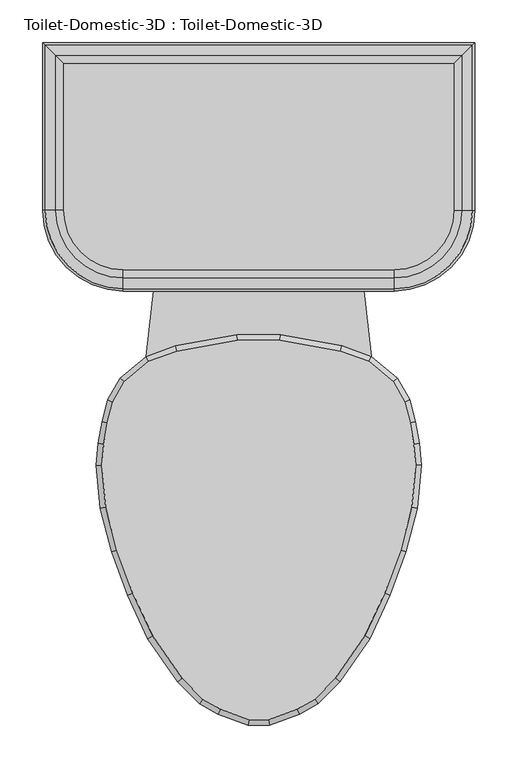
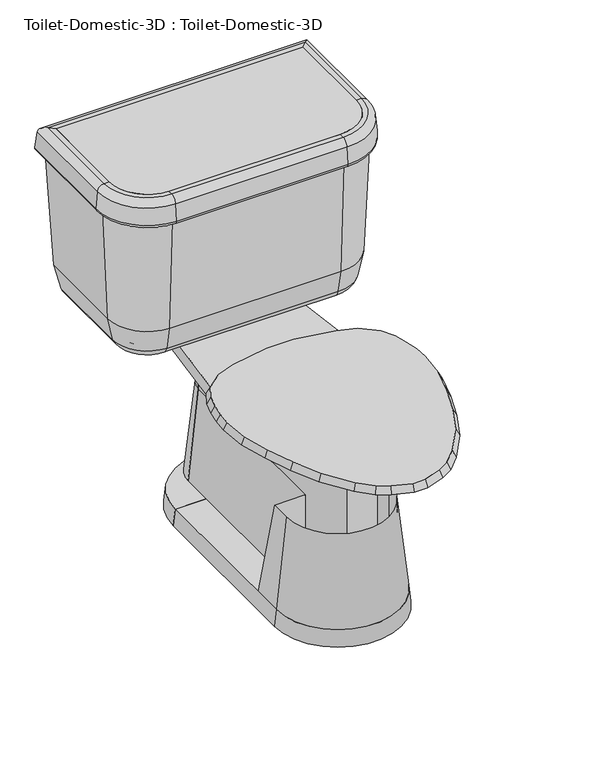
"""IFC4 building model written with IfcOpenShell, lengths in millimetres: flow terminal geometry, Toilet-Domestic-3D : Toilet-Domestic-3D."""

from ifc_helpers import new_model, si_unit, point, frame, frame_2d, origin, place, context, project, spatial, polyline, circle_curve, ellipse_curve, trimmed, segment, composite_curve, outline, extrude, faceted_brep, source, transform, mapped, element, save
from ifc_brep_helpers import plane_surface, cylinder_surface, revolved_surface, advanced_brep


def toilet_domestic_3d_toilet_domestic_3d_f7549cf7(model_context):
    return source(origin(), model_context, "Body", "SolidModel", [
        advanced_brep(
        [(-117.7636364, 285.75, 0.0), (-38.1, 285.75, 0.0), (-38.1, 285.75, 31.75), (-114.3, 285.75, 31.75), (117.7636364, 285.75, 0.0), (114.3, 285.75, 31.75), (38.1, 285.75, 31.75), (38.1, 285.75, 0.0)],
        [
            (0, 1),
            (1, 2),
            (2, 3),
            (3, 0),
            (4, 5),
            (5, 6),
            (6, 7),
            (7, 4),
            (7, 1, circle_curve(frame((0.0, 285.75, 0.0), z_axis=(0.0, 0.0, 1.0), x_axis=(-1.0, 0.0, 0.0)), 38.1)),
            (0, 4, circle_curve(frame((0.0, 285.75, 0.0), z_axis=(0.0, 0.0, -1.0), x_axis=(-1.0, 0.0, 0.0)), 117.7636364)),
            (6, 2, circle_curve(frame((0.0, 285.75, 31.75), z_axis=(0.0, 0.0, 1.0), x_axis=(-1.0, 0.0, 0.0)), 38.1)),
            (5, 3, circle_curve(frame((0.0, 285.75, 31.75), z_axis=(0.0, 0.0, 1.0), x_axis=(-1.0, 0.0, 0.0)), 114.3)),
        ],
        [
            plane_surface(frame((0.0, 285.75, -304.8), z_axis=(0.0, -1.0, 0.0), x_axis=(-1.0, 0.0, 0.0))),
            plane_surface(frame((0.0, 285.75, -304.8), z_axis=(0.0, -1.0, 0.0), x_axis=(1.0, 0.0, 0.0))),
            plane_surface(frame((0.0, 285.75, 0.0), z_axis=(0.0, 0.0, -1.0), x_axis=(-1.0, 0.0, 0.0))),
            revolved_surface(polyline([(-38.1, 285.75, 0.0), (-38.1, 285.75, 31.75)]), (0.0, 285.75, -304.8), (0.0, 0.0, -1.0)),
            plane_surface(frame((0.0, 285.75, 31.75), z_axis=(0.0, 0.0, 1.0), x_axis=(-1.0, 0.0, 0.0))),
            revolved_surface(polyline([(-114.3, 285.75, 31.75), (-117.7636364, 285.75, 0.0)]), (0.0, 285.75, -304.8), (0.0, 0.0, -1.0)),
        ],
        [
            (0, [[1, 2, 3, 4]]),
            (1, [[5, 6, 7, 8]]),
            (2, [[9, -1, 10, -8]]),
            (3, [[11, -2, -9, -7]]),
            (4, [[12, -3, -11, -6]]),
            (5, [[-10, -4, -12, -5]]),
        ],
    ),
        advanced_brep(
        [(-38.1, 342.9, 206.375), (-57.15, 342.9, 31.75), (-38.1, 342.9, 31.75), (38.1, 342.9, 206.375), (38.1, 342.9, 31.75), (57.15, 342.9, 31.75)],
        [
            (0, 1),
            (1, 2),
            (2, 0),
            (3, 4),
            (4, 5),
            (5, 3),
            (5, 1, circle_curve(frame((0.0, 342.9, 31.75), z_axis=(0.0, 0.0, 1.0), x_axis=(-1.0, 0.0, 0.0)), 57.15)),
            (0, 3, circle_curve(frame((0.0, 342.9, 206.375), z_axis=(0.0, 0.0, -1.0), x_axis=(-1.0, 0.0, 0.0)), 38.1)),
            (4, 2, circle_curve(frame((0.0, 342.9, 31.75), z_axis=(0.0, 0.0, 1.0), x_axis=(-1.0, 0.0, 0.0)), 38.1)),
        ],
        [
            plane_surface(frame((0.0, 342.9, 31.75), z_axis=(0.0, -1.0, 0.0), x_axis=(-1.0, 0.0, 0.0))),
            plane_surface(frame((0.0, 342.9, 31.75), z_axis=(0.0, -1.0, 0.0), x_axis=(1.0, 0.0, 0.0))),
            revolved_surface(polyline([(-38.1, 342.9, 206.375), (-57.15, 342.9, 31.75)]), (0.0, 342.9, 31.75), (0.0, 0.0, -1.0)),
            plane_surface(frame((0.0, 342.9, 31.75), z_axis=(0.0, 0.0, -1.0), x_axis=(-1.0, 0.0, 0.0))),
            revolved_surface(polyline([(-38.1, 342.9, 31.75), (-38.1, 342.9, 206.375)]), (0.0, 342.9, 31.75), (0.0, 0.0, -1.0)),
        ],
        [
            (0, [[1, 2, 3]]),
            (1, [[4, 5, 6]]),
            (2, [[7, -1, 8, -6]]),
            (3, [[9, -2, -7, -5]]),
            (4, [[-8, -3, -9, -4]]),
        ],
    ),
        faceted_brep([(-157.6293435, 97.472128, 400.05), (-171.060664, 73.773864, 400.05), (-177.5851102, 49.4242991, 400.05), (-181.9845715, 24.4737144, 400.05), (-184.125744, 0.0, 400.05), (-179.7950716, -49.4998127, 400.05), (-166.347, -99.688699, 400.05), (-148.0469602, -149.9676451, 400.05), (-124.7045808, -200.0255393, 400.05), (-90.0971582, -249.9125941, 400.05), (-65.691017, -274.3187354, 400.05), (-44.8990862, -286.3229622, 400.05), (-11.5803237, -298.45, 400.05), (11.5803237, -298.45, 400.05), (44.8990862, -286.3229622, 400.05), (65.691017, -274.3187354, 400.05), (90.0971582, -249.9125941, 400.05), (124.7045808, -200.0255393, 400.05), (148.0469602, -149.9676451, 400.05), (166.347, -99.688699, 400.05), (179.7950716, -49.4998127, 400.05), (184.125744, 0.0, 400.05), (181.9845715, 24.4737144, 400.05), (177.5851102, 49.4242991, 400.05), (171.060664, 73.773864, 400.05), (157.6293435, 97.472128, 400.05), (129.0942628, 121.4159037, 400.05), (95.7755003, 133.5429415, 400.05), (24.844447, 146.05, 400.05), (-24.844447, 146.05, 400.05), (-95.7755003, 133.5429415, 400.05), (-129.0942628, 121.4159037, 400.05), (-162.5887836, 101.6, 387.2181453), (-132.3182423, 127.0, 387.2181453), (-97.4252791, 139.7, 387.2181453), (-25.4, 152.4, 387.2181453), (25.4, 152.4, 387.2181453), (97.4252791, 139.7, 387.2181453), (132.3182423, 127.0, 387.2181453), (162.5887836, 101.6, 387.2181453), (176.9845865, 76.2, 387.2181453), (183.790496, 50.8, 387.2181453), (188.2862441, 25.3033453, 387.2181453), (190.5, 0.0, 387.2181453), (186.0724883, -50.6066907, 387.2181453), (172.4088722, -101.6, 387.2181453), (153.9191843, -152.4, 387.2181453), (130.2307553, -203.2, 387.2181453), (94.9900085, -254.0, 387.2181453), (69.5900085, -279.4, 387.2181453), (47.5929632, -292.1, 387.2181453), (12.7, -304.8, 387.2181453), (-12.7, -304.8, 387.2181453), (-47.5929632, -292.1, 387.2181453), (-69.5900085, -279.4, 387.2181453), (-94.9900085, -254.0, 387.2181453), (-130.2307553, -203.2, 387.2181453), (-153.9191843, -152.4, 387.2181453), (-172.4088722, -101.6, 387.2181453), (-186.0724883, -50.6066907, 387.2181453), (-190.5, 0.0, 387.2181453), (-188.2862441, 25.3033453, 387.2181453), (-183.790496, 50.8, 387.2181453), (-176.9845865, 76.2, 387.2181453)], [[[0, 1, 2, 3, 4, 5, 6, 7, 8, 9, 10, 11, 12, 13, 14, 15, 16, 17, 18, 19, 20, 21, 22, 23, 24, 25, 26, 27, 28, 29, 30, 31]], [[32, 33, 34, 35, 36, 37, 38, 39, 40, 41, 42, 43, 44, 45, 46, 47, 48, 49, 50, 51, 52, 53, 54, 55, 56, 57, 58, 59, 60, 61, 62, 63]], [[32, 63, 1, 0]], [[63, 62, 2, 1]], [[62, 61, 3, 2]], [[61, 60, 4, 3]], [[60, 59, 5, 4]], [[59, 58, 6, 5]], [[58, 57, 7, 6]], [[57, 56, 8, 7]], [[56, 55, 9, 8]], [[55, 54, 10, 9]], [[54, 53, 11, 10]], [[53, 52, 12, 11]], [[52, 51, 13, 12]], [[51, 50, 14, 13]], [[50, 49, 15, 14]], [[49, 48, 16, 15]], [[48, 47, 17, 16]], [[47, 46, 18, 17]], [[46, 45, 19, 18]], [[45, 44, 20, 19]], [[44, 43, 21, 20]], [[43, 42, 22, 21]], [[42, 41, 23, 22]], [[41, 40, 24, 23]], [[40, 39, 25, 24]], [[39, 38, 26, 25]], [[38, 37, 27, 26]], [[37, 36, 28, 27]], [[36, 35, 29, 28]], [[35, 34, 30, 29]], [[34, 33, 31, 30]], [[33, 32, 0, 31]]]),
        extrude(outline(composite_curve([segment(polyline([(228.5868869, 469.8868869), (228.5868869, 298.45)]), True, "CONTINUOUS"), segment(trimmed(circle_curve(frame_2d((158.75, 298.45)), 69.8368869), [point((228.5868869, 298.45))], [point((158.75, 228.6131131))], False, "CARTESIAN"), True, "CONTINUOUS"), segment(polyline([(158.75, 228.6131131), (-158.75, 228.6131131)]), True, "CONTINUOUS"), segment(trimmed(circle_curve(frame_2d((-158.75, 298.45)), 69.8368869), [point((-158.75, 228.6131131))], [point((-228.5868869, 298.45))], False, "CARTESIAN"), True, "CONTINUOUS"), segment(polyline([(-228.5868869, 298.45), (-228.5868869, 469.8868869), (228.5868869, 469.8868869)]), True, "CONTINUOUS")], self_intersect=False)), frame((0.0, 0.0, 654.05), z_axis=(0.0, 0.0, 1.0), x_axis=(1.0, 0.0, 0.0)), (0.0, 0.0, 1.0), 50.8),
        extrude(outline(composite_curve([segment(trimmed(circle_curve(frame_2d((0.0, 342.9)), 38.1), [point((-38.1, 342.9))], [point((38.1, 342.9))], False, "CARTESIAN"), True, "CONTINUOUS"), segment(polyline([(38.1, 342.9), (-38.1, 342.9)]), True, "CONTINUOUS")], self_intersect=False)), frame((0.0, 0.0, 206.375), z_axis=(0.0, 0.0, 1.0), x_axis=(1.0, 0.0, 0.0)), (0.0, 0.0, 1.0), 130.175),
        advanced_brep(
        [(177.8, 419.1, 387.2181453), (177.8, 419.1, 374.65), (177.8, 298.45, 374.65), (177.8, 298.45, 387.2181453), (192.8020829, 434.1020829, 387.2181453), (192.8020829, 298.45, 387.2181453), (211.4650931, 452.7650931, 402.4478636), (211.4650931, 298.45, 402.4478636), (218.7732506, 460.0732506, 438.15), (218.7732506, 298.45, 438.15), (228.5868869, 469.8868869, 654.05), (228.5868869, 298.45, 654.05), (228.5868869, 469.8868869, 704.85), (228.5868869, 298.45, 704.85), (237.91817, 479.21817, 704.85), (237.91817, 298.45, 704.85), (250.5698426, 491.8698426, 693.2568779), (250.5698426, 298.45, 693.2568779), (253.3960274, 494.6960274, 660.953439), (253.3960274, 298.45, 660.953439), (247.070191, 488.370191, 654.05), (247.070191, 298.45, 654.05), (241.3, 482.6, 654.05), (241.3, 298.45, 654.05), (231.4863636, 472.7863636, 438.15), (231.4863636, 298.45, 438.15), (222.3416824, 463.6416824, 393.4759963), (222.3416824, 298.45, 393.4759963), (197.8071664, 439.1071664, 374.65), (197.8071664, 298.45, 374.65), (158.75, 279.4, 387.2181453), (158.75, 279.4, 374.65), (158.75, 264.3979171, 387.2181453), (158.75, 245.7349069, 402.4478636), (158.75, 238.4267494, 438.15), (158.75, 228.6131131, 654.05), (158.75, 228.6131131, 704.85), (158.75, 219.28183, 704.85), (158.75, 206.6301574, 693.2568779), (158.75, 203.8039726, 660.953439), (158.75, 210.129809, 654.05), (158.75, 215.9, 654.05), (158.75, 225.7136364, 438.15), (158.75, 234.8583176, 393.4759963), (158.75, 259.3928336, 374.65), (-158.75, 279.4, 374.65), (-158.75, 279.4, 387.2181453), (-158.75, 264.3979171, 387.2181453), (-158.75, 245.7349069, 402.4478636), (-158.75, 238.4267494, 438.15), (-158.75, 228.6131131, 654.05), (-158.75, 228.6131131, 704.85), (-158.75, 219.28183, 704.85), (-158.75, 206.6301574, 693.2568779), (-158.75, 203.8039726, 660.953439), (-158.75, 210.129809, 654.05), (-158.75, 215.9, 654.05), (-158.75, 225.7136364, 438.15), (-158.75, 234.8583176, 393.4759963), (-158.75, 259.3928336, 374.65), (-177.8, 298.45, 387.2181453), (-177.8, 298.45, 374.65), (-192.8020829, 298.45, 387.2181453), (-211.4650931, 298.45, 402.4478636), (-218.7732506, 298.45, 438.15), (-228.5868869, 298.45, 654.05), (-228.5868869, 298.45, 704.85), (-237.91817, 298.45, 704.85), (-250.5698426, 298.45, 693.2568779), (-253.3960274, 298.45, 660.953439), (-247.070191, 298.45, 654.05), (-241.3, 298.45, 654.05), (-231.4863636, 298.45, 438.15), (-222.3416824, 298.45, 393.4759963), (-197.8071664, 298.45, 374.65), (-177.8, 419.1, 374.65), (-177.8, 419.1, 387.2181453), (-192.8020829, 434.1020829, 387.2181453), (-211.4650931, 452.7650931, 402.4478636), (-218.7732506, 460.0732506, 438.15), (-228.5868869, 469.8868869, 654.05), (-228.5868869, 469.8868869, 704.85), (-237.91817, 479.21817, 704.85), (-250.5698426, 491.8698426, 693.2568779), (-253.3960274, 494.6960274, 660.953439), (-247.070191, 488.370191, 654.05), (-241.3, 482.6, 654.05), (-231.4863636, 472.7863636, 438.15), (-222.3416824, 463.6416824, 393.4759963), (-197.8071664, 439.1071664, 374.65)],
        [
            (0, 1),
            (1, 2),
            (2, 3),
            (3, 0),
            (4, 0),
            (3, 5),
            (5, 4),
            (6, 4, ellipse_curve(frame((192.8020829, 434.1020829, 406.2681453), z_axis=(-0.7071067811865451, 0.7071067811865498, 0.0), x_axis=(-0.7071067811865497, -0.7071067811865452, 0.0)), 26.9407684, 19.05)),
            (5, 7, circle_curve(frame((192.8020829, 298.45, 406.2681453), z_axis=(0.0, -1.0, 0.0), x_axis=(1.0, 0.0, 0.0)), 19.05)),
            (7, 6),
            (8, 6),
            (7, 9),
            (9, 8),
            (10, 8),
            (9, 11),
            (11, 10),
            (12, 10),
            (11, 13),
            (13, 12),
            (14, 12),
            (13, 15),
            (15, 14),
            (16, 14, ellipse_curve(frame((237.91817, 479.21817, 692.15), z_axis=(0.7071067811865451, -0.7071067811865498, 0.0), x_axis=(0.7071067811865497, 0.7071067811865452, 0.0)), 17.9605122, 12.7)),
            (15, 17, circle_curve(frame((237.91817, 298.45, 692.15), z_axis=(0.0, 1.0, 0.0), x_axis=(1.0, 0.0, 0.0)), 12.7)),
            (17, 16),
            (18, 16),
            (17, 19),
            (19, 18),
            (20, 18, ellipse_curve(frame((247.070191, 488.370191, 660.4), z_axis=(0.7071067811865451, -0.7071067811865498, 0.0), x_axis=(0.7071067811865497, 0.7071067811865452, 0.0)), 8.9802561, 6.35)),
            (19, 21, circle_curve(frame((247.070191, 298.45, 660.4), z_axis=(0.0, 1.0, 0.0), x_axis=(1.0, 0.0, 0.0)), 6.35)),
            (21, 20),
            (22, 20),
            (21, 23),
            (23, 22),
            (24, 22),
            (23, 25),
            (25, 24),
            (26, 24),
            (25, 27),
            (27, 26),
            (28, 26, ellipse_curve(frame((197.8071664, 439.1071664, 400.05), z_axis=(0.7071067811865451, -0.7071067811865498, 0.0), x_axis=(0.7071067811865497, 0.7071067811865452, 0.0)), 35.9210245, 25.4)),
            (27, 29, circle_curve(frame((197.8071664, 298.45, 400.05), z_axis=(0.0, 1.0, 0.0), x_axis=(1.0, 0.0, 0.0)), 25.4)),
            (29, 28),
            (1, 28),
            (29, 2),
            (30, 3, circle_curve(frame((158.75, 298.45, 387.2181453), z_axis=(0.0, 0.0, 1.0), x_axis=(1.0, 0.0, 0.0)), 19.05)),
            (2, 31, circle_curve(frame((158.75, 298.45, 374.65), z_axis=(0.0, 0.0, -1.0), x_axis=(1.0, 0.0, 0.0)), 19.05)),
            (31, 30),
            (32, 5, circle_curve(frame((158.75, 298.45, 387.2181453), z_axis=(0.0, 0.0, 1.0), x_axis=(1.0, 0.0, 0.0)), 34.0520829)),
            (30, 32),
            (33, 7, circle_curve(frame((158.75, 298.45, 402.4478636), z_axis=(0.0, 0.0, 1.0), x_axis=(1.0, 0.0, 0.0)), 52.7150931)),
            (32, 33, circle_curve(frame((158.75, 264.3979171, 406.2681453), z_axis=(-1.0, 0.0, 0.0), x_axis=(0.0, -1.0, 0.0)), 19.05)),
            (34, 9, circle_curve(frame((158.75, 298.45, 438.15), z_axis=(0.0, 0.0, 1.0), x_axis=(1.0, 0.0, 0.0)), 60.0232506)),
            (33, 34),
            (35, 11, circle_curve(frame((158.75, 298.45, 654.05), z_axis=(0.0, 0.0, 1.0), x_axis=(1.0, 0.0, 0.0)), 69.8368869)),
            (34, 35),
            (36, 13, circle_curve(frame((158.75, 298.45, 704.85), z_axis=(0.0, 0.0, 1.0), x_axis=(1.0, 0.0, 0.0)), 69.8368869)),
            (35, 36),
            (37, 15, circle_curve(frame((158.75, 298.45, 704.85), z_axis=(0.0, 0.0, 1.0), x_axis=(1.0, 0.0, 0.0)), 79.16817)),
            (36, 37),
            (38, 17, circle_curve(frame((158.75, 298.45, 693.2568779), z_axis=(0.0, 0.0, 1.0), x_axis=(1.0, 0.0, 0.0)), 91.8198426)),
            (37, 38, circle_curve(frame((158.75, 219.28183, 692.15), z_axis=(1.0, 0.0, 0.0), x_axis=(0.0, -1.0, 0.0)), 12.7)),
            (39, 19, circle_curve(frame((158.75, 298.45, 660.953439), z_axis=(0.0, 0.0, 1.0), x_axis=(1.0, 0.0, 0.0)), 94.6460274)),
            (38, 39),
            (40, 21, circle_curve(frame((158.75, 298.45, 654.05), z_axis=(0.0, 0.0, 1.0), x_axis=(1.0, 0.0, 0.0)), 88.320191)),
            (39, 40, circle_curve(frame((158.75, 210.129809, 660.4), z_axis=(1.0, 0.0, 0.0), x_axis=(0.0, -1.0, 0.0)), 6.35)),
            (41, 23, circle_curve(frame((158.75, 298.45, 654.05), z_axis=(0.0, 0.0, 1.0), x_axis=(1.0, 0.0, 0.0)), 82.55)),
            (40, 41),
            (42, 25, circle_curve(frame((158.75, 298.45, 438.15), z_axis=(0.0, 0.0, 1.0), x_axis=(1.0, 0.0, 0.0)), 72.7363636)),
            (41, 42),
            (43, 27, circle_curve(frame((158.75, 298.45, 393.4759963), z_axis=(0.0, 0.0, 1.0), x_axis=(1.0, 0.0, 0.0)), 63.5916824)),
            (42, 43),
            (44, 29, circle_curve(frame((158.75, 298.45, 374.65), z_axis=(0.0, 0.0, 1.0), x_axis=(1.0, 0.0, 0.0)), 39.0571664)),
            (43, 44, circle_curve(frame((158.75, 259.3928336, 400.05), z_axis=(1.0, 0.0, 0.0), x_axis=(0.0, -1.0, 0.0)), 25.4)),
            (44, 31),
            (31, 45),
            (45, 46),
            (46, 30),
            (46, 47),
            (47, 32),
            (47, 48, circle_curve(frame((-158.75, 264.3979171, 406.2681453), z_axis=(-1.0, 0.0, 0.0), x_axis=(0.0, -1.0, 0.0)), 19.05)),
            (48, 33),
            (48, 49),
            (49, 34),
            (49, 50),
            (50, 35),
            (50, 51),
            (51, 36),
            (51, 52),
            (52, 37),
            (52, 53, circle_curve(frame((-158.75, 219.28183, 692.15), z_axis=(1.0, 0.0, 0.0), x_axis=(0.0, -1.0, 0.0)), 12.7)),
            (53, 38),
            (53, 54),
            (54, 39),
            (54, 55, circle_curve(frame((-158.75, 210.129809, 660.4), z_axis=(1.0, 0.0, 0.0), x_axis=(0.0, -1.0, 0.0)), 6.35)),
            (55, 40),
            (55, 56),
            (56, 41),
            (56, 57),
            (57, 42),
            (57, 58),
            (58, 43),
            (58, 59, circle_curve(frame((-158.75, 259.3928336, 400.05), z_axis=(1.0, 0.0, 0.0), x_axis=(0.0, -1.0, 0.0)), 25.4)),
            (59, 44),
            (59, 45),
            (60, 46, circle_curve(frame((-158.75, 298.45, 387.2181453), z_axis=(0.0, 0.0, 1.0), x_axis=(0.0, -1.0, 0.0)), 19.05)),
            (45, 61, circle_curve(frame((-158.75, 298.45, 374.65), z_axis=(0.0, 0.0, -1.0), x_axis=(0.0, -1.0, 0.0)), 19.05)),
            (61, 60),
            (62, 47, circle_curve(frame((-158.75, 298.45, 387.2181453), z_axis=(0.0, 0.0, 1.0), x_axis=(0.0, -1.0, 0.0)), 34.0520829)),
            (60, 62),
            (63, 48, circle_curve(frame((-158.75, 298.45, 402.4478636), z_axis=(0.0, 0.0, 1.0), x_axis=(0.0, -1.0, 0.0)), 52.7150931)),
            (62, 63, circle_curve(frame((-192.8020829, 298.45, 406.2681453), z_axis=(0.0, 1.0, 0.0), x_axis=(-1.0, 0.0, 0.0)), 19.05)),
            (64, 49, circle_curve(frame((-158.75, 298.45, 438.15), z_axis=(0.0, 0.0, 1.0), x_axis=(0.0, -1.0, 0.0)), 60.0232506)),
            (63, 64),
            (65, 50, circle_curve(frame((-158.75, 298.45, 654.05), z_axis=(0.0, 0.0, 1.0), x_axis=(0.0, -1.0, 0.0)), 69.8368869)),
            (64, 65),
            (66, 51, circle_curve(frame((-158.75, 298.45, 704.85), z_axis=(0.0, 0.0, 1.0), x_axis=(0.0, -1.0, 0.0)), 69.8368869)),
            (65, 66),
            (67, 52, circle_curve(frame((-158.75, 298.45, 704.85), z_axis=(0.0, 0.0, 1.0), x_axis=(0.0, -1.0, 0.0)), 79.16817)),
            (66, 67),
            (68, 53, circle_curve(frame((-158.75, 298.45, 693.2568779), z_axis=(0.0, 0.0, 1.0), x_axis=(0.0, -1.0, 0.0)), 91.8198426)),
            (67, 68, circle_curve(frame((-237.91817, 298.45, 692.15), z_axis=(0.0, -1.0, 0.0), x_axis=(-1.0, 0.0, 0.0)), 12.7)),
            (69, 54, circle_curve(frame((-158.75, 298.45, 660.953439), z_axis=(0.0, 0.0, 1.0), x_axis=(0.0, -1.0, 0.0)), 94.6460274)),
            (68, 69),
            (70, 55, circle_curve(frame((-158.75, 298.45, 654.05), z_axis=(0.0, 0.0, 1.0), x_axis=(0.0, -1.0, 0.0)), 88.320191)),
            (69, 70, circle_curve(frame((-247.070191, 298.45, 660.4), z_axis=(0.0, -1.0, 0.0), x_axis=(-1.0, 0.0, 0.0)), 6.35)),
            (71, 56, circle_curve(frame((-158.75, 298.45, 654.05), z_axis=(0.0, 0.0, 1.0), x_axis=(0.0, -1.0, 0.0)), 82.55)),
            (70, 71),
            (72, 57, circle_curve(frame((-158.75, 298.45, 438.15), z_axis=(0.0, 0.0, 1.0), x_axis=(0.0, -1.0, 0.0)), 72.7363636)),
            (71, 72),
            (73, 58, circle_curve(frame((-158.75, 298.45, 393.4759963), z_axis=(0.0, 0.0, 1.0), x_axis=(0.0, -1.0, 0.0)), 63.5916824)),
            (72, 73),
            (74, 59, circle_curve(frame((-158.75, 298.45, 374.65), z_axis=(0.0, 0.0, 1.0), x_axis=(0.0, -1.0, 0.0)), 39.0571664)),
            (73, 74, circle_curve(frame((-197.8071664, 298.45, 400.05), z_axis=(0.0, -1.0, 0.0), x_axis=(-1.0, 0.0, 0.0)), 25.4)),
            (74, 61),
            (61, 75),
            (75, 76),
            (76, 60),
            (76, 77),
            (77, 62),
            (77, 78, ellipse_curve(frame((-192.8020829, 434.1020829, 406.2681453), z_axis=(0.7071067811865498, 0.7071067811865451, 0.0), x_axis=(-0.7071067811865451, 0.70710678118655, 0.0)), 26.9407684, 19.05)),
            (78, 63),
            (78, 79),
            (79, 64),
            (79, 80),
            (80, 65),
            (80, 81),
            (81, 66),
            (81, 82),
            (82, 67),
            (82, 83, ellipse_curve(frame((-237.91817, 479.21817, 692.15), z_axis=(-0.7071067811865498, -0.7071067811865451, 0.0), x_axis=(0.7071067811865451, -0.70710678118655, 0.0)), 17.9605122, 12.7)),
            (83, 68),
            (83, 84),
            (84, 69),
            (84, 85, ellipse_curve(frame((-247.070191, 488.370191, 660.4), z_axis=(-0.7071067811865498, -0.7071067811865451, 0.0), x_axis=(0.7071067811865451, -0.70710678118655, 0.0)), 8.9802561, 6.35)),
            (85, 70),
            (85, 86),
            (86, 71),
            (86, 87),
            (87, 72),
            (87, 88),
            (88, 73),
            (88, 89, ellipse_curve(frame((-197.8071664, 439.1071664, 400.05), z_axis=(-0.7071067811865498, -0.7071067811865451, 0.0), x_axis=(0.7071067811865451, -0.70710678118655, 0.0)), 35.9210245, 25.4)),
            (89, 74),
            (89, 75),
            (75, 1),
            (0, 76),
            (4, 77),
            (6, 78),
            (8, 79),
            (10, 80),
            (12, 81),
            (14, 82),
            (16, 83),
            (18, 84),
            (20, 85),
            (22, 86),
            (24, 87),
            (26, 88),
            (28, 89),
        ],
        [
            plane_surface(frame((177.8, 419.1, 374.65), z_axis=(-1.0, 0.0, 0.0), x_axis=(0.0, -1.0, 0.0))),
            plane_surface(frame((177.8, 419.1, 387.2181453), z_axis=(0.0, 0.0, 1.0), x_axis=(0.0, -1.0, 0.0))),
            revolved_surface(polyline([(211.8520829, 298.45, 406.2681453), (211.8520829, 453.1520829260162, 406.2681453)]), (192.8020829, 419.1, 406.2681453), (0.0, -1.0, 0.0)),
            plane_surface(frame((211.4650931, 452.7650931, 402.4478636), z_axis=(-0.9796855721787505, 0.0, 0.2005397209153197), x_axis=(0.0, -1.0, 0.0))),
            plane_surface(frame((218.7732506, 460.0732506, 438.15), z_axis=(-0.9989685402102995, 0.0, 0.045407660918654086), x_axis=(0.0, -1.0, 0.0))),
            plane_surface(frame((228.5868869, 469.8868869, 654.05), z_axis=(-1.0, 0.0, 0.0), x_axis=(0.0, -1.0, 0.0))),
            plane_surface(frame((228.5868869, 469.8868869, 704.85), z_axis=(0.0, 0.0, 1.0), x_axis=(0.0, -1.0, 0.0))),
            cylinder_surface(frame((237.91817, 419.1, 692.15), z_axis=(0.0, 1.0, 0.0), x_axis=(1.0, 0.0, 0.0)), 12.7),
            plane_surface(frame((250.5698426, 491.8698426, 693.2568779), z_axis=(0.9961946980917452, 0.0, 0.08715574274766269), x_axis=(0.0, -1.0, 0.0))),
            cylinder_surface(frame((247.070191, 419.1, 660.4), z_axis=(0.0, 1.0, 0.0), x_axis=(1.0, 0.0, 0.0)), 6.35),
            plane_surface(frame((247.070191, 488.370191, 654.05), z_axis=(0.0, 0.0, -1.0), x_axis=(0.0, -1.0, 0.0))),
            plane_surface(frame((241.3, 482.6, 654.05), z_axis=(0.9989685402102993, 0.0, -0.04540766091865594), x_axis=(0.0, -1.0, 0.0))),
            plane_surface(frame((231.4863636, 472.7863636, 438.15), z_axis=(0.9796855721787489, 0.0, -0.20053972091532798), x_axis=(0.0, -1.0, 0.0))),
            cylinder_surface(frame((197.8071664, 419.1, 400.05), z_axis=(0.0, 1.0, 0.0), x_axis=(1.0, 0.0, 0.0)), 25.4),
            plane_surface(frame((197.8071664, 439.1071664, 374.65), z_axis=(0.0, 0.0, -1.0), x_axis=(0.0, -1.0, 0.0))),
            revolved_surface(polyline([(177.8, 298.45, 374.65), (177.8, 298.45, 387.2181453)]), (158.75, 298.45, 0.0), (0.0, 0.0, -1.0)),
            plane_surface(frame((158.75, 298.45, 387.2181453), z_axis=(0.0, 0.0, 1.0), x_axis=(1.0, 0.0, 0.0))),
            revolved_surface(trimmed(ellipse_curve(frame((192.8020829, 298.45, 406.2681453), z_axis=(0.0, -1.0, 0.0), x_axis=(1.0, 0.0, 0.0)), 19.05, 19.05), [point((192.8020829, 298.45, 387.2181453))], [point((211.4650931, 298.45, 402.4478636))], True, "CARTESIAN"), (158.75, 298.45, 0.0), (0.0, 0.0, -1.0)),
            revolved_surface(polyline([(211.4650931, 298.45, 402.4478636), (218.7732506, 298.45, 438.15)]), (158.75, 298.45, 0.0), (0.0, 0.0, -1.0)),
            revolved_surface(polyline([(218.7732506, 298.45, 438.15), (228.5868869, 298.45, 654.05)]), (158.75, 298.45, 0.0), (0.0, 0.0, -1.0)),
            revolved_surface(polyline([(228.5868869, 298.45, 654.05), (228.5868869, 298.45, 704.85)]), (158.75, 298.45, 0.0), (0.0, 0.0, -1.0)),
            plane_surface(frame((158.75, 298.45, 704.85), z_axis=(0.0, 0.0, 1.0), x_axis=(1.0, 0.0, 0.0))),
            revolved_surface(trimmed(ellipse_curve(frame((237.91817, 298.45, 692.15), z_axis=(0.0, 1.0, 0.0), x_axis=(1.0, 0.0, 0.0)), 12.7, 12.7), [point((237.91817, 298.45, 704.85))], [point((250.5698426, 298.45, 693.2568779))], True, "CARTESIAN"), (158.75, 298.45, 0.0), (0.0, 0.0, -1.0)),
            revolved_surface(polyline([(250.5698426, 298.45, 693.2568779), (253.3960274, 298.45, 660.953439)]), (158.75, 298.45, 0.0), (0.0, 0.0, -1.0)),
            revolved_surface(trimmed(ellipse_curve(frame((247.070191, 298.45, 660.4), z_axis=(0.0, 1.0, 0.0), x_axis=(1.0, 0.0, 0.0)), 6.35, 6.35), [point((253.3960274, 298.45, 660.953439))], [point((247.070191, 298.45, 654.05))], True, "CARTESIAN"), (158.75, 298.45, 0.0), (0.0, 0.0, -1.0)),
            plane_surface(frame((158.75, 298.45, 654.05), z_axis=(0.0, 0.0, -1.0), x_axis=(1.0, 0.0, 0.0))),
            revolved_surface(polyline([(241.3, 298.45, 654.05), (231.4863636, 298.45, 438.15)]), (158.75, 298.45, 0.0), (0.0, 0.0, -1.0)),
            revolved_surface(polyline([(231.4863636, 298.45, 438.15), (222.3416824, 298.45, 393.4759963)]), (158.75, 298.45, 0.0), (0.0, 0.0, -1.0)),
            revolved_surface(trimmed(ellipse_curve(frame((197.8071664, 298.45, 400.05), z_axis=(0.0, 1.0, 0.0), x_axis=(1.0, 0.0, 0.0)), 25.4, 25.4), [point((222.3416824, 298.45, 393.4759963))], [point((197.8071664, 298.45, 374.65))], True, "CARTESIAN"), (158.75, 298.45, 0.0), (0.0, 0.0, -1.0)),
            plane_surface(frame((158.75, 298.45, 374.65), z_axis=(0.0, 0.0, -1.0), x_axis=(1.0, 0.0, 0.0))),
            plane_surface(frame((158.75, 279.4, 374.65), z_axis=(0.0, 1.0, 0.0), x_axis=(-1.0, 0.0, 0.0))),
            plane_surface(frame((158.75, 279.4, 387.2181453), z_axis=(0.0, 0.0, 1.0), x_axis=(-1.0, 0.0, 0.0))),
            revolved_surface(polyline([(-158.75, 245.34791709999996, 406.2681453), (158.75, 245.34791709999996, 406.2681453)]), (158.75, 264.3979171, 406.2681453), (-1.0, 0.0, 0.0)),
            plane_surface(frame((158.75, 245.7349069, 402.4478636), z_axis=(0.0, 0.9796855721787505, 0.2005397209153197), x_axis=(-1.0, 0.0, 0.0))),
            plane_surface(frame((158.75, 238.4267494, 438.15), z_axis=(0.0, 0.9989685402102995, 0.045407660918654086), x_axis=(-1.0, 0.0, 0.0))),
            plane_surface(frame((158.75, 228.6131131, 654.05), z_axis=(0.0, 1.0, 0.0), x_axis=(-1.0, 0.0, 0.0))),
            plane_surface(frame((158.75, 228.6131131, 704.85), z_axis=(0.0, 0.0, 1.0), x_axis=(-1.0, 0.0, 0.0))),
            cylinder_surface(frame((158.75, 219.28183, 692.15), z_axis=(1.0, 0.0, 0.0), x_axis=(0.0, -1.0, 0.0)), 12.7),
            plane_surface(frame((158.75, 206.6301574, 693.2568779), z_axis=(0.0, -0.9961946980917452, 0.08715574274766269), x_axis=(-1.0, 0.0, 0.0))),
            cylinder_surface(frame((158.75, 210.129809, 660.4), z_axis=(1.0, 0.0, 0.0), x_axis=(0.0, -1.0, 0.0)), 6.35),
            plane_surface(frame((158.75, 210.129809, 654.05), z_axis=(0.0, 0.0, -1.0), x_axis=(-1.0, 0.0, 0.0))),
            plane_surface(frame((158.75, 215.9, 654.05), z_axis=(0.0, -0.9989685402102993, -0.04540766091865594), x_axis=(-1.0, 0.0, 0.0))),
            plane_surface(frame((158.75, 225.7136364, 438.15), z_axis=(0.0, -0.9796855721787489, -0.20053972091532798), x_axis=(-1.0, 0.0, 0.0))),
            cylinder_surface(frame((158.75, 259.3928336, 400.05), z_axis=(1.0, 0.0, 0.0), x_axis=(0.0, -1.0, 0.0)), 25.4),
            plane_surface(frame((158.75, 259.3928336, 374.65), z_axis=(0.0, 0.0, -1.0), x_axis=(-1.0, 0.0, 0.0))),
            revolved_surface(polyline([(-158.75, 279.4, 374.65), (-158.75, 279.4, 387.2181453)]), (-158.75, 298.45, 0.0), (0.0, 0.0, -1.0)),
            plane_surface(frame((-158.75, 298.45, 387.2181453), z_axis=(0.0, 0.0, 1.0), x_axis=(0.0, -1.0, 0.0))),
            revolved_surface(trimmed(ellipse_curve(frame((-158.75, 264.3979171, 406.2681453), z_axis=(-1.0, 0.0, 0.0), x_axis=(0.0, -1.0, 0.0)), 19.05, 19.05), [point((-158.75, 264.3979171, 387.2181453))], [point((-158.75, 245.7349069, 402.4478636))], True, "CARTESIAN"), (-158.75, 298.45, 0.0), (0.0, 0.0, -1.0)),
            revolved_surface(polyline([(-158.75, 245.7349069, 402.4478636), (-158.75, 238.4267494, 438.15)]), (-158.75, 298.45, 0.0), (0.0, 0.0, -1.0)),
            revolved_surface(polyline([(-158.75, 238.4267494, 438.15), (-158.75, 228.6131131, 654.05)]), (-158.75, 298.45, 0.0), (0.0, 0.0, -1.0)),
            revolved_surface(polyline([(-158.75, 228.6131131, 654.05), (-158.75, 228.6131131, 704.85)]), (-158.75, 298.45, 0.0), (0.0, 0.0, -1.0)),
            plane_surface(frame((-158.75, 298.45, 704.85), z_axis=(0.0, 0.0, 1.0), x_axis=(0.0, -1.0, 0.0))),
            revolved_surface(trimmed(ellipse_curve(frame((-158.75, 219.28183, 692.15), z_axis=(1.0, 0.0, 0.0), x_axis=(0.0, -1.0, 0.0)), 12.7, 12.7), [point((-158.75, 219.28183, 704.85))], [point((-158.75, 206.6301574, 693.2568779))], True, "CARTESIAN"), (-158.75, 298.45, 0.0), (0.0, 0.0, -1.0)),
            revolved_surface(polyline([(-158.75, 206.6301574, 693.2568779), (-158.75, 203.8039726, 660.953439)]), (-158.75, 298.45, 0.0), (0.0, 0.0, -1.0)),
            revolved_surface(trimmed(ellipse_curve(frame((-158.75, 210.129809, 660.4), z_axis=(1.0, 0.0, 0.0), x_axis=(0.0, -1.0, 0.0)), 6.35, 6.35), [point((-158.75, 203.8039726, 660.953439))], [point((-158.75, 210.129809, 654.05))], True, "CARTESIAN"), (-158.75, 298.45, 0.0), (0.0, 0.0, -1.0)),
            plane_surface(frame((-158.75, 298.45, 654.05), z_axis=(0.0, 0.0, -1.0), x_axis=(0.0, -1.0, 0.0))),
            revolved_surface(polyline([(-158.75, 215.9, 654.05), (-158.75, 225.7136364, 438.15)]), (-158.75, 298.45, 0.0), (0.0, 0.0, -1.0)),
            revolved_surface(polyline([(-158.75, 225.7136364, 438.15), (-158.75, 234.8583176, 393.4759963)]), (-158.75, 298.45, 0.0), (0.0, 0.0, -1.0)),
            revolved_surface(trimmed(ellipse_curve(frame((-158.75, 259.3928336, 400.05), z_axis=(1.0, 0.0, 0.0), x_axis=(0.0, -1.0, 0.0)), 25.4, 25.4), [point((-158.75, 234.8583176, 393.4759963))], [point((-158.75, 259.3928336, 374.65))], True, "CARTESIAN"), (-158.75, 298.45, 0.0), (0.0, 0.0, -1.0)),
            plane_surface(frame((-158.75, 298.45, 374.65), z_axis=(0.0, 0.0, -1.0), x_axis=(0.0, -1.0, 0.0))),
            plane_surface(frame((-177.8, 298.45, 374.65), z_axis=(1.0, 0.0, 0.0), x_axis=(0.0, 1.0, 0.0))),
            plane_surface(frame((-177.8, 298.45, 387.2181453), z_axis=(0.0, 0.0, 1.0), x_axis=(0.0, 1.0, 0.0))),
            revolved_surface(polyline([(-211.8520829, 453.15208292601636, 406.2681453), (-211.8520829, 298.45, 406.2681453)]), (-192.8020829, 298.45, 406.2681453), (0.0, 1.0, 0.0)),
            plane_surface(frame((-211.4650931, 298.45, 402.4478636), z_axis=(0.9796855721787505, 0.0, 0.2005397209153197), x_axis=(0.0, 1.0, 0.0))),
            plane_surface(frame((-218.7732506, 298.45, 438.15), z_axis=(0.9989685402102995, 0.0, 0.045407660918654086), x_axis=(0.0, 1.0, 0.0))),
            plane_surface(frame((-228.5868869, 298.45, 654.05), z_axis=(1.0, 0.0, 0.0), x_axis=(0.0, 1.0, 0.0))),
            plane_surface(frame((-228.5868869, 298.45, 704.85), z_axis=(0.0, 0.0, 1.0), x_axis=(0.0, 1.0, 0.0))),
            cylinder_surface(frame((-237.91817, 298.45, 692.15), z_axis=(0.0, -1.0, 0.0), x_axis=(-1.0, 0.0, 0.0)), 12.7),
            plane_surface(frame((-250.5698426, 298.45, 693.2568779), z_axis=(-0.9961946980917452, 0.0, 0.08715574274766269), x_axis=(0.0, 1.0, 0.0))),
            cylinder_surface(frame((-247.070191, 298.45, 660.4), z_axis=(0.0, -1.0, 0.0), x_axis=(-1.0, 0.0, 0.0)), 6.35),
            plane_surface(frame((-247.070191, 298.45, 654.05), z_axis=(0.0, 0.0, -1.0), x_axis=(0.0, 1.0, 0.0))),
            plane_surface(frame((-241.3, 298.45, 654.05), z_axis=(-0.9989685402102993, 0.0, -0.04540766091865594), x_axis=(0.0, 1.0, 0.0))),
            plane_surface(frame((-231.4863636, 298.45, 438.15), z_axis=(-0.9796855721787489, 0.0, -0.20053972091532798), x_axis=(0.0, 1.0, 0.0))),
            cylinder_surface(frame((-197.8071664, 298.45, 400.05), z_axis=(0.0, -1.0, 0.0), x_axis=(-1.0, 0.0, 0.0)), 25.4),
            plane_surface(frame((-197.8071664, 298.45, 374.65), z_axis=(0.0, 0.0, -1.0), x_axis=(0.0, 1.0, 0.0))),
            plane_surface(frame((-177.8, 419.1, 374.65), z_axis=(0.0, -1.0, 0.0), x_axis=(1.0, 0.0, 0.0))),
            plane_surface(frame((-177.8, 419.1, 387.2181453), z_axis=(0.0, 0.0, 1.0), x_axis=(1.0, 0.0, 0.0))),
            revolved_surface(polyline([(211.85208292601635, 453.15208290000004, 406.2681453), (-211.85208292601618, 453.15208290000004, 406.2681453)]), (-177.8, 434.1020829, 406.2681453), (1.0, 0.0, 0.0)),
            plane_surface(frame((-211.4650931, 452.7650931, 402.4478636), z_axis=(0.0, -0.9796855721787505, 0.2005397209153197), x_axis=(1.0, 0.0, 0.0))),
            plane_surface(frame((-218.7732506, 460.0732506, 438.15), z_axis=(0.0, -0.9989685402102995, 0.045407660918654086), x_axis=(1.0, 0.0, 0.0))),
            plane_surface(frame((-228.5868869, 469.8868869, 654.05), z_axis=(0.0, -1.0, 0.0), x_axis=(1.0, 0.0, 0.0))),
            plane_surface(frame((-228.5868869, 469.8868869, 704.85), z_axis=(0.0, 0.0, 1.0), x_axis=(1.0, 0.0, 0.0))),
            cylinder_surface(frame((-177.8, 479.21817, 692.15), z_axis=(-1.0, 0.0, 0.0), x_axis=(0.0, 1.0, 0.0)), 12.7),
            plane_surface(frame((-250.5698426, 491.8698426, 693.2568779), z_axis=(0.0, 0.9961946980917452, 0.08715574274766269), x_axis=(1.0, 0.0, 0.0))),
            cylinder_surface(frame((-177.8, 488.370191, 660.4), z_axis=(-1.0, 0.0, 0.0), x_axis=(0.0, 1.0, 0.0)), 6.35),
            plane_surface(frame((-247.070191, 488.370191, 654.05), z_axis=(0.0, 0.0, -1.0), x_axis=(1.0, 0.0, 0.0))),
            plane_surface(frame((-241.3, 482.6, 654.05), z_axis=(0.0, 0.9989685402102993, -0.04540766091865594), x_axis=(1.0, 0.0, 0.0))),
            plane_surface(frame((-231.4863636, 472.7863636, 438.15), z_axis=(0.0, 0.9796855721787489, -0.20053972091532798), x_axis=(1.0, 0.0, 0.0))),
            cylinder_surface(frame((-177.8, 439.1071664, 400.05), z_axis=(-1.0, 0.0, 0.0), x_axis=(0.0, 1.0, 0.0)), 25.4),
            plane_surface(frame((-197.8071664, 439.1071664, 374.65), z_axis=(0.0, 0.0, -1.0), x_axis=(1.0, 0.0, 0.0))),
        ],
        [
            (0, [[1, 2, 3, 4]]),
            (1, [[5, -4, 6, 7]]),
            (2, [[8, -7, 9, 10]]),
            (3, [[11, -10, 12, 13]]),
            (4, [[14, -13, 15, 16]]),
            (5, [[17, -16, 18, 19]]),
            (6, [[20, -19, 21, 22]]),
            (7, [[23, -22, 24, 25]]),
            (8, [[26, -25, 27, 28]]),
            (9, [[29, -28, 30, 31]]),
            (10, [[32, -31, 33, 34]]),
            (11, [[35, -34, 36, 37]]),
            (12, [[38, -37, 39, 40]]),
            (13, [[41, -40, 42, 43]]),
            (14, [[44, -43, 45, -2]]),
            (15, [[46, -3, 47, 48]]),
            (16, [[49, -6, -46, 50]]),
            (17, [[51, -9, -49, 52]]),
            (18, [[53, -12, -51, 54]]),
            (19, [[55, -15, -53, 56]]),
            (20, [[57, -18, -55, 58]]),
            (21, [[59, -21, -57, 60]]),
            (22, [[61, -24, -59, 62]]),
            (23, [[63, -27, -61, 64]]),
            (24, [[65, -30, -63, 66]]),
            (25, [[67, -33, -65, 68]]),
            (26, [[69, -36, -67, 70]]),
            (27, [[71, -39, -69, 72]]),
            (28, [[73, -42, -71, 74]]),
            (29, [[-47, -45, -73, 75]]),
            (30, [[-48, 76, 77, 78]]),
            (31, [[-50, -78, 79, 80]]),
            (32, [[-52, -80, 81, 82]]),
            (33, [[-54, -82, 83, 84]]),
            (34, [[-56, -84, 85, 86]]),
            (35, [[-58, -86, 87, 88]]),
            (36, [[-60, -88, 89, 90]]),
            (37, [[-62, -90, 91, 92]]),
            (38, [[-64, -92, 93, 94]]),
            (39, [[-66, -94, 95, 96]]),
            (40, [[-68, -96, 97, 98]]),
            (41, [[-70, -98, 99, 100]]),
            (42, [[-72, -100, 101, 102]]),
            (43, [[-74, -102, 103, 104]]),
            (44, [[-75, -104, 105, -76]]),
            (45, [[106, -77, 107, 108]]),
            (46, [[109, -79, -106, 110]]),
            (47, [[111, -81, -109, 112]]),
            (48, [[113, -83, -111, 114]]),
            (49, [[115, -85, -113, 116]]),
            (50, [[117, -87, -115, 118]]),
            (51, [[119, -89, -117, 120]]),
            (52, [[121, -91, -119, 122]]),
            (53, [[123, -93, -121, 124]]),
            (54, [[125, -95, -123, 126]]),
            (55, [[127, -97, -125, 128]]),
            (56, [[129, -99, -127, 130]]),
            (57, [[131, -101, -129, 132]]),
            (58, [[133, -103, -131, 134]]),
            (59, [[-107, -105, -133, 135]]),
            (60, [[-108, 136, 137, 138]]),
            (61, [[-110, -138, 139, 140]]),
            (62, [[-112, -140, 141, 142]]),
            (63, [[-114, -142, 143, 144]]),
            (64, [[-116, -144, 145, 146]]),
            (65, [[-118, -146, 147, 148]]),
            (66, [[-120, -148, 149, 150]]),
            (67, [[-122, -150, 151, 152]]),
            (68, [[-124, -152, 153, 154]]),
            (69, [[-126, -154, 155, 156]]),
            (70, [[-128, -156, 157, 158]]),
            (71, [[-130, -158, 159, 160]]),
            (72, [[-132, -160, 161, 162]]),
            (73, [[-134, -162, 163, 164]]),
            (74, [[-135, -164, 165, -136]]),
            (75, [[-137, 166, -1, 167]]),
            (76, [[-139, -167, -5, 168]]),
            (77, [[-141, -168, -8, 169]]),
            (78, [[-143, -169, -11, 170]]),
            (79, [[-145, -170, -14, 171]]),
            (80, [[-147, -171, -17, 172]]),
            (81, [[-149, -172, -20, 173]]),
            (82, [[-151, -173, -23, 174]]),
            (83, [[-153, -174, -26, 175]]),
            (84, [[-155, -175, -29, 176]]),
            (85, [[-157, -176, -32, 177]]),
            (86, [[-159, -177, -35, 178]]),
            (87, [[-161, -178, -38, 179]]),
            (88, [[-163, -179, -41, 180]]),
            (89, [[-165, -180, -44, -166]]),
        ],
    ),
        extrude(outline(composite_curve([segment(polyline([(-25.4, 152.4), (-97.4252791, 139.7), (-132.3182423, 127.0), (-101.4824733, 395.1508638)]), True, "CONTINUOUS"), segment(trimmed(circle_curve(frame_2d((-88.8656197, 393.7)), 12.7), [point((-101.4824733, 395.1508638))], [point((-88.8656197, 406.4))], False, "CARTESIAN"), True, "CONTINUOUS"), segment(polyline([(-88.8656197, 406.4), (88.8656197, 406.4)]), True, "CONTINUOUS"), segment(trimmed(circle_curve(frame_2d((88.8656197, 393.7)), 12.7), [point((88.8656197, 406.4))], [point((101.4824733, 395.1508638))], False, "CARTESIAN"), True, "CONTINUOUS"), segment(polyline([(101.4824733, 395.1508638), (132.3182423, 127.0), (97.4252791, 139.7), (25.4, 152.4), (0.0, 152.4), (-25.4, 152.4)]), True, "CONTINUOUS")], self_intersect=False)), frame((0.0, 0.0, 336.55), z_axis=(0.0, 0.0, 1.0), x_axis=(1.0, 0.0, 0.0)), (0.0, 0.0, 1.0), 25.4),
        extrude(outline(polyline([(139.7, 264.5247209), (152.4, 336.55), (342.9, 336.55), (342.9, 206.375), (107.4852632, 206.375), (127.0, 229.6317577), (139.7, 264.5247209)])), frame((-38.1, 0.0, 0.0), z_axis=(1.0, 0.0, 0.0), x_axis=(0.0, 1.0, 0.0)), (0.0, 0.0, 1.0), 76.2),
        advanced_brep(
        [(-117.7636364, 285.75, 0.0), (-114.3, 285.75, 31.75), (-38.1, 285.75, 31.75), (-38.1, 285.75, 0.0), (-117.7636364, -38.0999951, 0.0), (-114.3, -38.0999951, 31.75), (-38.1, -38.0999951, 31.75), (-38.1, -38.0999951, 0.0), (114.2999707, -38.0999951, 31.75), (117.7636071, -38.0999951, 0.0), (38.0999707, -38.0999951, 31.75), (38.0999707, -38.0999951, 0.0), (117.7636071, 285.6681634, 0.0), (38.0999707, 285.6681634, 0.0), (38.0999707, 285.6681634, 31.75), (114.2999707, 285.6681634, 31.75)],
        [
            (0, 1),
            (1, 2),
            (2, 3),
            (3, 0),
            (0, 4),
            (4, 5),
            (5, 1),
            (5, 6),
            (6, 2),
            (6, 7),
            (7, 3),
            (7, 4),
            (8, 5, circle_curve(frame((-1.46e-05, -38.0999951, 31.75), z_axis=(0.0, 0.0, -1.0), x_axis=(-1.0, 0.0, 0.0)), 114.2999854)),
            (4, 9, circle_curve(frame((-1.46e-05, -38.0999951, 0.0), z_axis=(0.0, 0.0, 1.0), x_axis=(-1.0, 0.0, 0.0)), 117.7636217)),
            (9, 8),
            (10, 6, circle_curve(frame((-1.46e-05, -38.0999951, 31.75), z_axis=(0.0, 0.0, -1.0), x_axis=(-1.0, 0.0, 0.0)), 38.0999854)),
            (8, 10),
            (11, 7, circle_curve(frame((-1.46e-05, -38.0999951, 0.0), z_axis=(0.0, 0.0, -1.0), x_axis=(-1.0, 0.0, 0.0)), 38.0999854)),
            (10, 11),
            (11, 9),
            (12, 13),
            (13, 14),
            (14, 15),
            (15, 12),
            (9, 12),
            (15, 8),
            (14, 10),
            (13, 11),
        ],
        [
            plane_surface(frame((-196.85, 285.75, 0.0), z_axis=(0.0, 1.0, 0.0), x_axis=(0.0, 0.0, -1.0))),
            plane_surface(frame((-117.7636364, 285.75, 0.0), z_axis=(-0.9941021766079929, 0.0, 0.10844751017543448), x_axis=(0.0, -1.0, 0.0))),
            plane_surface(frame((-114.3, 285.75, 31.75), z_axis=(0.0, 0.0, 1.0), x_axis=(0.0, -1.0, 0.0))),
            plane_surface(frame((-38.1, 285.75, 31.75), z_axis=(1.0, 0.0, 0.0), x_axis=(0.0, -1.0, 0.0))),
            plane_surface(frame((-38.1, 285.75, 0.0), z_axis=(0.0, 0.0, -1.0), x_axis=(0.0, -1.0, 0.0))),
            revolved_surface(polyline([(-117.7636364, -38.0999951, 0.0), (-114.3, -38.0999951, 31.75)]), (-1.46e-05, -38.0999951, 0.0), (0.0, 0.0, 1.0)),
            plane_surface(frame((-1.46e-05, -38.0999951, 31.75), z_axis=(0.0, 0.0, 1.0), x_axis=(-1.0, 0.0, 0.0))),
            revolved_surface(polyline([(-38.1, -38.0999951, 31.75), (-38.1, -38.0999951, 0.0)]), (-1.46e-05, -38.0999951, 0.0), (0.0, 0.0, 1.0)),
            plane_surface(frame((-1.46e-05, -38.0999951, 0.0), z_axis=(0.0, 0.0, -1.0), x_axis=(-1.0, 0.0, 0.0))),
            plane_surface(frame((31.7499707, 285.6681634, 0.0), z_axis=(0.0, 1.0, 0.0), x_axis=(0.0, 0.0, 1.0))),
            plane_surface(frame((117.7636071, -38.0999951, 0.0), z_axis=(0.9941021766079929, 0.0, 0.10844751017543448), x_axis=(0.0, 1.0, 0.0))),
            plane_surface(frame((114.2999707, -38.0999951, 31.75), z_axis=(0.0, 0.0, 1.0), x_axis=(0.0, 1.0, 0.0))),
            plane_surface(frame((38.0999707, -38.0999951, 31.75), z_axis=(-1.0, 0.0, 0.0), x_axis=(0.0, 1.0, 0.0))),
            plane_surface(frame((38.0999707, -38.0999951, 0.0), z_axis=(0.0, 0.0, -1.0), x_axis=(0.0, 1.0, 0.0))),
        ],
        [
            (0, [[1, 2, 3, 4]]),
            (1, [[-1, 5, 6, 7]]),
            (2, [[-2, -7, 8, 9]]),
            (3, [[-3, -9, 10, 11]]),
            (4, [[-4, -11, 12, -5]]),
            (5, [[13, -6, 14, 15]]),
            (6, [[16, -8, -13, 17]]),
            (7, [[18, -10, -16, 19]]),
            (8, [[-14, -12, -18, 20]]),
            (9, [[21, 22, 23, 24]]),
            (10, [[-15, 25, -24, 26]]),
            (11, [[-17, -26, -23, 27]]),
            (12, [[-19, -27, -22, 28]]),
            (13, [[-20, -28, -21, -25]]),
        ],
    ),
        advanced_brep(
        [(-57.15, 342.9, 31.75), (-38.1, 342.9, 206.375), (-38.1, 342.9, 31.75), (-57.15, 19.05, 31.75), (-38.1, 0.0, 206.375), (-38.1, 0.0, 31.75), (-114.3, 19.05, 31.75), (-95.25, 0.0, 206.375), (-95.25, 0.0, 31.75), (-114.3, -38.1, 31.75), (-95.25, -38.1, 206.375), (-95.25, -38.1, 31.75), (95.25, -38.1, 206.375), (114.3, -38.1, 31.75), (95.25, -38.1, 31.75), (114.3, 19.05, 31.75), (95.25, 0.0, 206.375), (95.25, 0.0, 31.75), (57.15, 19.05, 31.75), (38.1, 0.0, 206.375), (38.1, 0.0, 31.75), (57.15, 342.9, 31.75), (38.1, 342.9, 31.75), (38.1, 342.9, 206.375)],
        [
            (0, 1),
            (1, 2),
            (2, 0),
            (0, 3),
            (3, 4),
            (4, 1),
            (4, 5),
            (5, 2),
            (5, 3),
            (3, 6),
            (6, 7),
            (7, 4),
            (7, 8),
            (8, 5),
            (8, 6),
            (6, 9),
            (9, 10),
            (10, 7),
            (10, 11),
            (11, 8),
            (11, 9),
            (12, 10, circle_curve(frame((0.0, -38.1, 206.375), z_axis=(0.0, 0.0, -1.0), x_axis=(-1.0, 0.0, 0.0)), 95.25)),
            (9, 13, circle_curve(frame((0.0, -38.1, 31.75), z_axis=(0.0, 0.0, 1.0), x_axis=(-1.0, 0.0, 0.0)), 114.3)),
            (13, 12),
            (14, 11, circle_curve(frame((0.0, -38.1, 31.75), z_axis=(0.0, 0.0, -1.0), x_axis=(-1.0, 0.0, 0.0)), 95.25)),
            (12, 14),
            (14, 13),
            (13, 15),
            (15, 16),
            (16, 12),
            (16, 17),
            (17, 14),
            (17, 15),
            (15, 18),
            (18, 19),
            (19, 16),
            (19, 20),
            (20, 17),
            (20, 18),
            (21, 22),
            (22, 23),
            (23, 21),
            (18, 21),
            (23, 19),
            (22, 20),
        ],
        [
            plane_surface(frame((-244.475, 342.9, 0.0), z_axis=(0.0, 1.0, 0.0), x_axis=(0.0, 0.0, -1.0))),
            plane_surface(frame((-57.15, 342.9, 31.75), z_axis=(-0.9941021766079944, 0.0, 0.10844751017542063), x_axis=(0.0, -1.0, 0.0))),
            plane_surface(frame((-38.1, 342.9, 206.375), z_axis=(1.0, 0.0, 0.0), x_axis=(0.0, -1.0, 0.0))),
            plane_surface(frame((-38.1, 342.9, 31.75), z_axis=(0.0, 0.0, -1.0), x_axis=(0.0, -1.0, 0.0))),
            plane_surface(frame((-57.15, 19.05, 31.75), z_axis=(0.0, 0.9941021766079944, 0.10844751017542063), x_axis=(-1.0, 0.0, 0.0))),
            plane_surface(frame((-38.1, 0.0, 206.375), z_axis=(0.0, -1.0, 0.0), x_axis=(-1.0, 0.0, 0.0))),
            plane_surface(frame((-38.1, 0.0, 31.75), z_axis=(0.0, 0.0, -1.0), x_axis=(-1.0, 0.0, 0.0))),
            plane_surface(frame((-114.3, 19.05, 31.75), z_axis=(-0.9941021766079944, 0.0, 0.10844751017542063), x_axis=(0.0, -1.0, 0.0))),
            plane_surface(frame((-95.25, 0.0, 206.375), z_axis=(1.0, 0.0, 0.0), x_axis=(0.0, -1.0, 0.0))),
            plane_surface(frame((-95.25, 0.0, 31.75), z_axis=(0.0, 0.0, -1.0), x_axis=(0.0, -1.0, 0.0))),
            revolved_surface(polyline([(-114.3, -38.1, 31.75), (-95.25, -38.1, 206.375)]), (0.0, -38.1, 0.0), (0.0, 0.0, 1.0)),
            revolved_surface(polyline([(-95.25, -38.1, 206.375), (-95.25, -38.1, 31.75)]), (0.0, -38.1, 0.0), (0.0, 0.0, 1.0)),
            plane_surface(frame((0.0, -38.1, 31.75), z_axis=(0.0, 0.0, -1.0), x_axis=(-1.0, 0.0, 0.0))),
            plane_surface(frame((114.3, -38.1, 31.75), z_axis=(0.9941021766079944, 0.0, 0.10844751017542063), x_axis=(0.0, 1.0, 0.0))),
            plane_surface(frame((95.25, -38.1, 206.375), z_axis=(-1.0, 0.0, 0.0), x_axis=(0.0, 1.0, 0.0))),
            plane_surface(frame((95.25, -38.1, 31.75), z_axis=(0.0, 0.0, -1.0), x_axis=(0.0, 1.0, 0.0))),
            plane_surface(frame((114.3, 19.05, 31.75), z_axis=(0.0, 0.9941021766079944, 0.10844751017542063), x_axis=(-1.0, 0.0, 0.0))),
            plane_surface(frame((95.25, 0.0, 206.375), z_axis=(0.0, -1.0, 0.0), x_axis=(-1.0, 0.0, 0.0))),
            plane_surface(frame((95.25, 0.0, 31.75), z_axis=(0.0, 0.0, -1.0), x_axis=(-1.0, 0.0, 0.0))),
            plane_surface(frame((-168.275, 342.9, 0.0), z_axis=(0.0, 1.0, 0.0), x_axis=(0.0, 0.0, 1.0))),
            plane_surface(frame((57.15, 19.05, 31.75), z_axis=(0.9941021766079944, 0.0, 0.10844751017542063), x_axis=(0.0, 1.0, 0.0))),
            plane_surface(frame((38.1, 0.0, 206.375), z_axis=(-1.0, 0.0, 0.0), x_axis=(0.0, 1.0, 0.0))),
            plane_surface(frame((38.1, 0.0, 31.75), z_axis=(0.0, 0.0, -1.0), x_axis=(0.0, 1.0, 0.0))),
        ],
        [
            (0, [[1, 2, 3]]),
            (1, [[-1, 4, 5, 6]]),
            (2, [[-2, -6, 7, 8]]),
            (3, [[-3, -8, 9, -4]]),
            (4, [[-5, 10, 11, 12]]),
            (5, [[-7, -12, 13, 14]]),
            (6, [[-9, -14, 15, -10]]),
            (7, [[-11, 16, 17, 18]]),
            (8, [[-13, -18, 19, 20]]),
            (9, [[-15, -20, 21, -16]]),
            (10, [[22, -17, 23, 24]]),
            (11, [[25, -19, -22, 26]]),
            (12, [[-23, -21, -25, 27]]),
            (13, [[-24, 28, 29, 30]]),
            (14, [[-26, -30, 31, 32]]),
            (15, [[-27, -32, 33, -28]]),
            (16, [[-29, 34, 35, 36]]),
            (17, [[-31, -36, 37, 38]]),
            (18, [[-33, -38, 39, -34]]),
            (19, [[40, 41, 42]]),
            (20, [[-35, 43, -42, 44]]),
            (21, [[-37, -44, -41, 45]]),
            (22, [[-39, -45, -40, -43]]),
        ],
    ),
    ])


if __name__ == "__main__":
    model = new_model("IFC4")
    model_context = context("Model", 3, world=origin())
    ifc_project = project(units=[si_unit("LENGTHUNIT", "METRE", prefix="MILLI")], contexts=[model_context])
    site = spatial("IfcSite", under=ifc_project)
    building = spatial("IfcBuilding", under=site)
    placement = place(None, origin())
    toilet_domestic_3d_toilet_domestic_3d_shape = toilet_domestic_3d_toilet_domestic_3d_f7549cf7(model_context)
    element("IfcFlowTerminal", 1, ObjectType="Toilet-Domestic-3D : Toilet-Domestic-3D", at=placement, inside=building, context=model_context, shape_type="MappedRepresentation", body=[
        mapped(toilet_domestic_3d_toilet_domestic_3d_shape, transform((0.0, 0.0, 0.0), x_axis=(1.0, 0.0, 0.0), y_axis=(0.0, 1.0, 0.0), z_axis=(0.0, 0.0, 1.0))),
    ])
    save(model, "model.ifc")

# Revit data of these elements
# Type "Toilet-Domestic-3D : Toilet-Domestic-3D"
#   Assembly Code = "D2010110"
#   Toilet - Bowl/Basin Material = Porcelain, Linen
#   Toilet - Seat Material = Laminate, Linen, Matte
# Element 1 (IfcFlowTerminal, "Toilet-Domestic-3D : Toilet-Domestic-3D")
#   Materials on its faces: "Porcelain, Linen", "Laminate, Linen, Matte"
# Materials
#   "Porcelain, Linen": class "Ceramic", colour RGB 249 239 230, transparency 0, Description = "Porcelain, linen", Cost = 0
#   "Laminate, Linen, Matte": class "Plastic", colour RGB 249 239 230, transparency 0, Description = "Plastic Laminate - Linen, Matte", Cost = 0
